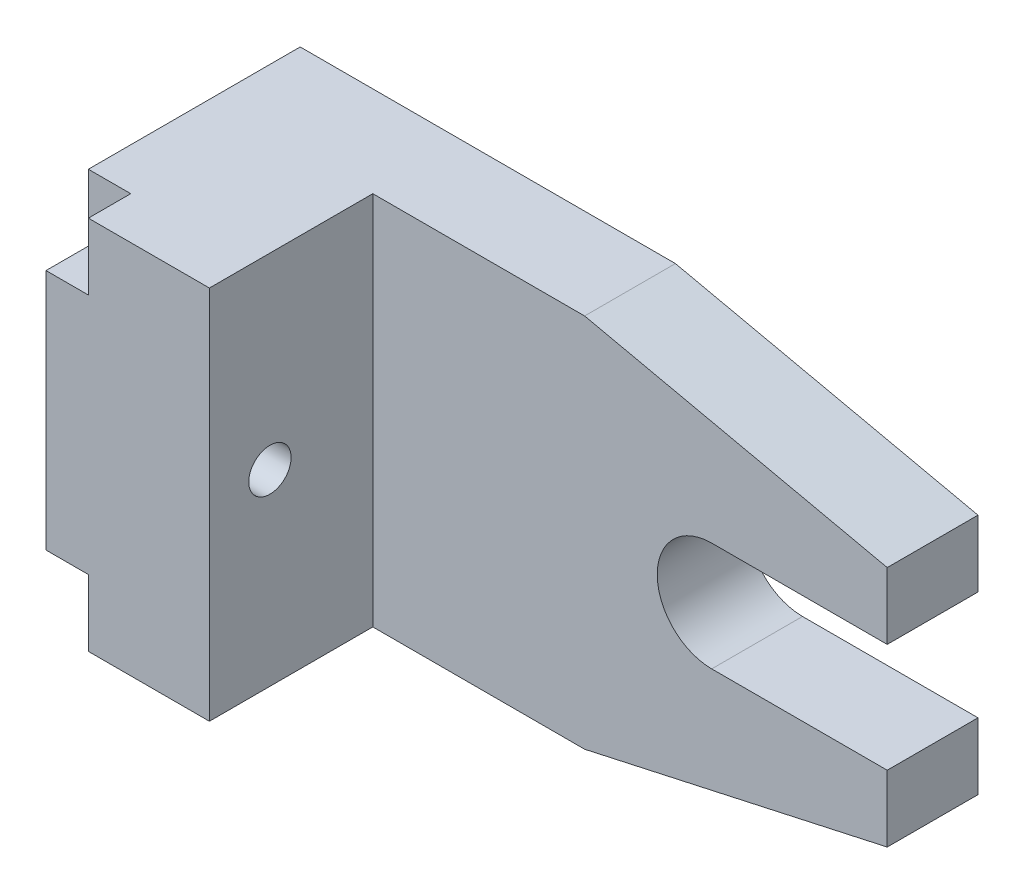
ISO-10303-21;
HEADER;
FILE_DESCRIPTION(('STEP AP214'),'2;1');
FILE_NAME('part.step','',(''),(''),'','','');
FILE_SCHEMA(('AUTOMOTIVE_DESIGN { 1 0 10303 214 1 1 1 1 }'));
ENDSEC;
DATA;
#1=APPLICATION_CONTEXT('core data for automotive mechanical design processes');
#2=APPLICATION_PROTOCOL_DEFINITION('international standard','automotive_design',2000,#1);
#3=PRODUCT_CONTEXT('',#1,'mechanical');
#4=PRODUCT('Part','Part','',(#3));
#5=PRODUCT_RELATED_PRODUCT_CATEGORY('part','',(#4));
#6=PRODUCT_DEFINITION_FORMATION('','',#4);
#7=PRODUCT_DEFINITION_CONTEXT('part definition',#1,'design');
#8=PRODUCT_DEFINITION('design','',#6,#7);
#9=PRODUCT_DEFINITION_SHAPE('','',#8);
#10=(LENGTH_UNIT() NAMED_UNIT(*) SI_UNIT(.MILLI.,.METRE.));
#11=(NAMED_UNIT(*) PLANE_ANGLE_UNIT() SI_UNIT($,.RADIAN.));
#12=(NAMED_UNIT(*) SI_UNIT($,.STERADIAN.) SOLID_ANGLE_UNIT());
#13=UNCERTAINTY_MEASURE_WITH_UNIT(LENGTH_MEASURE(1.E-05),#10,'distance_accuracy_value','');
#14=(GEOMETRIC_REPRESENTATION_CONTEXT(3) GLOBAL_UNCERTAINTY_ASSIGNED_CONTEXT((#13)) GLOBAL_UNIT_ASSIGNED_CONTEXT((#10,
#11,#12)) REPRESENTATION_CONTEXT('',''));
#15=CARTESIAN_POINT('',(0.,0.,0.));
#16=DIRECTION('',(0.,0.,1.));
#17=DIRECTION('',(1.,0.,0.));
#18=AXIS2_PLACEMENT_3D('',#15,#16,#17);
#19=CARTESIAN_POINT('',(0.,62.,15.));
#20=DIRECTION('',(0.,1.,0.));
#21=DIRECTION('',(0.,0.,1.));
#22=AXIS2_PLACEMENT_3D('',#19,#20,#21);
#23=PLANE('',#22);
#24=DIRECTION('',(0.,0.,-1.));
#25=VECTOR('',#24,1.);
#26=CARTESIAN_POINT('',(-27.,62.,42.));
#27=LINE('',#26,#25);
#28=CARTESIAN_POINT('',(-27.,62.,35.));
#29=VERTEX_POINT('',#28);
#30=CARTESIAN_POINT('',(-27.,62.,0.));
#31=VERTEX_POINT('',#30);
#32=EDGE_CURVE('E239',#29,#31,#27,.T.);
#33=ORIENTED_EDGE('',*,*,#32,.F.);
#34=DIRECTION('',(-1.,0.,0.));
#35=VECTOR('',#34,1.);
#36=CARTESIAN_POINT('',(-20.,62.,35.));
#37=LINE('',#36,#35);
#38=CARTESIAN_POINT('',(-20.,62.,35.));
#39=VERTEX_POINT('',#38);
#40=EDGE_CURVE('E196',#39,#29,#37,.T.);
#41=ORIENTED_EDGE('',*,*,#40,.F.);
#42=DIRECTION('',(0.,0.,-1.));
#43=VECTOR('',#42,1.);
#44=CARTESIAN_POINT('',(-20.,62.,0.));
#45=LINE('',#44,#43);
#46=CARTESIAN_POINT('',(-20.,62.,42.));
#47=VERTEX_POINT('',#46);
#48=EDGE_CURVE('E181',#47,#39,#45,.T.);
#49=ORIENTED_EDGE('',*,*,#48,.F.);
#50=DIRECTION('',(-1.,0.,0.));
#51=VECTOR('',#50,1.);
#52=CARTESIAN_POINT('',(0.,62.,42.));
#53=LINE('',#52,#51);
#54=CARTESIAN_POINT('',(0.,62.,42.));
#55=VERTEX_POINT('',#54);
#56=EDGE_CURVE('E221',#55,#47,#53,.T.);
#57=ORIENTED_EDGE('',*,*,#56,.F.);
#58=DIRECTION('',(0.,0.,-1.));
#59=VECTOR('',#58,1.);
#60=CARTESIAN_POINT('',(0.,62.,42.));
#61=LINE('',#60,#59);
#62=CARTESIAN_POINT('',(0.,62.,15.));
#63=VERTEX_POINT('',#62);
#64=EDGE_CURVE('E241',#55,#63,#61,.T.);
#65=ORIENTED_EDGE('',*,*,#64,.T.);
#66=DIRECTION('',(1.,0.,0.));
#67=VECTOR('',#66,1.);
#68=CARTESIAN_POINT('',(0.,62.,15.));
#69=LINE('',#68,#67);
#70=CARTESIAN_POINT('',(35.,62.,15.));
#71=VERTEX_POINT('',#70);
#72=EDGE_CURVE('E258',#63,#71,#69,.T.);
#73=ORIENTED_EDGE('',*,*,#72,.T.);
#74=DIRECTION('',(0.,0.,-1.));
#75=VECTOR('',#74,1.);
#76=CARTESIAN_POINT('',(35.,62.,15.));
#77=LINE('',#76,#75);
#78=CARTESIAN_POINT('',(35.,62.,0.));
#79=VERTEX_POINT('',#78);
#80=EDGE_CURVE('E303',#71,#79,#77,.T.);
#81=ORIENTED_EDGE('',*,*,#80,.T.);
#82=DIRECTION('',(1.,0.,0.));
#83=VECTOR('',#82,1.);
#84=CARTESIAN_POINT('',(0.,62.,0.));
#85=LINE('',#84,#83);
#86=EDGE_CURVE('E282',#31,#79,#85,.T.);
#87=ORIENTED_EDGE('',*,*,#86,.F.);
#88=EDGE_LOOP('',(#33,#41,#49,#57,#65,#73,#81,#87));
#89=FACE_BOUND('',#88,.T.);
#90=ADVANCED_FACE('F45',(#89),#23,.T.);
#91=CARTESIAN_POINT('',(0.,0.,15.));
#92=DIRECTION('',(0.,1.,0.));
#93=DIRECTION('',(0.,0.,1.));
#94=AXIS2_PLACEMENT_3D('',#91,#92,#93);
#95=PLANE('',#94);
#96=DIRECTION('',(-1.,0.,0.));
#97=VECTOR('',#96,1.);
#98=CARTESIAN_POINT('',(-20.,0.,35.));
#99=LINE('',#98,#97);
#100=CARTESIAN_POINT('',(-20.,0.,35.));
#101=VERTEX_POINT('',#100);
#102=CARTESIAN_POINT('',(-27.,0.,35.));
#103=VERTEX_POINT('',#102);
#104=EDGE_CURVE('E220',#101,#103,#99,.T.);
#105=ORIENTED_EDGE('',*,*,#104,.T.);
#106=DIRECTION('',(0.,0.,-1.));
#107=VECTOR('',#106,1.);
#108=CARTESIAN_POINT('',(-27.,0.,42.));
#109=LINE('',#108,#107);
#110=CARTESIAN_POINT('',(-27.,0.,0.));
#111=VERTEX_POINT('',#110);
#112=EDGE_CURVE('E240',#103,#111,#109,.T.);
#113=ORIENTED_EDGE('',*,*,#112,.T.);
#114=DIRECTION('',(1.,0.,0.));
#115=VECTOR('',#114,1.);
#116=CARTESIAN_POINT('',(0.,0.,0.));
#117=LINE('',#116,#115);
#118=CARTESIAN_POINT('',(35.,0.,0.));
#119=VERTEX_POINT('',#118);
#120=EDGE_CURVE('E285',#111,#119,#117,.T.);
#121=ORIENTED_EDGE('',*,*,#120,.T.);
#122=DIRECTION('',(0.,0.,-1.));
#123=VECTOR('',#122,1.);
#124=CARTESIAN_POINT('',(35.,0.,15.));
#125=LINE('',#124,#123);
#126=CARTESIAN_POINT('',(35.,0.,15.));
#127=VERTEX_POINT('',#126);
#128=EDGE_CURVE('E300',#127,#119,#125,.T.);
#129=ORIENTED_EDGE('',*,*,#128,.F.);
#130=DIRECTION('',(1.,0.,0.));
#131=VECTOR('',#130,1.);
#132=CARTESIAN_POINT('',(0.,0.,15.));
#133=LINE('',#132,#131);
#134=CARTESIAN_POINT('',(0.,0.,15.));
#135=VERTEX_POINT('',#134);
#136=EDGE_CURVE('E265',#135,#127,#133,.T.);
#137=ORIENTED_EDGE('',*,*,#136,.F.);
#138=DIRECTION('',(0.,0.,-1.));
#139=VECTOR('',#138,1.);
#140=CARTESIAN_POINT('',(0.,0.,42.));
#141=LINE('',#140,#139);
#142=CARTESIAN_POINT('',(0.,0.,42.));
#143=VERTEX_POINT('',#142);
#144=EDGE_CURVE('E235',#143,#135,#141,.T.);
#145=ORIENTED_EDGE('',*,*,#144,.F.);
#146=DIRECTION('',(1.,0.,0.));
#147=VECTOR('',#146,1.);
#148=CARTESIAN_POINT('',(-27.,0.,42.));
#149=LINE('',#148,#147);
#150=CARTESIAN_POINT('',(-20.,0.,42.));
#151=VERTEX_POINT('',#150);
#152=EDGE_CURVE('E230',#151,#143,#149,.T.);
#153=ORIENTED_EDGE('',*,*,#152,.F.);
#154=DIRECTION('',(0.,0.,1.));
#155=VECTOR('',#154,1.);
#156=CARTESIAN_POINT('',(-20.,0.,0.));
#157=LINE('',#156,#155);
#158=EDGE_CURVE('E67',#101,#151,#157,.T.);
#159=ORIENTED_EDGE('',*,*,#158,.F.);
#160=EDGE_LOOP('',(#105,#113,#121,#129,#137,#145,#153,#159));
#161=FACE_BOUND('',#160,.T.);
#162=ADVANCED_FACE('F342',(#161),#95,.F.);
#163=CARTESIAN_POINT('',(-27.,62.,42.));
#164=DIRECTION('',(1.,0.,0.));
#165=DIRECTION('',(0.,0.,-1.));
#166=AXIS2_PLACEMENT_3D('',#163,#164,#165);
#167=PLANE('',#166);
#168=CARTESIAN_POINT('',(-27.,31.,32.));
#169=DIRECTION('',(-1.,0.,0.));
#170=DIRECTION('',(0.,0.,1.));
#171=AXIS2_PLACEMENT_3D('',#168,#169,#170);
#172=CIRCLE('',#171,3.5);
#173=CARTESIAN_POINT('',(-27.,31.,35.5));
#174=VERTEX_POINT('',#173);
#175=EDGE_CURVE('E195',#174,#174,#172,.T.);
#176=ORIENTED_EDGE('',*,*,#175,.F.);
#177=EDGE_LOOP('',(#176));
#178=FACE_BOUND('',#177,.T.);
#179=DIRECTION('',(0.,1.,0.));
#180=VECTOR('',#179,1.);
#181=CARTESIAN_POINT('',(-27.,0.,35.));
#182=LINE('',#181,#180);
#183=CARTESIAN_POINT('',(-27.,51.,35.));
#184=VERTEX_POINT('',#183);
#185=EDGE_CURVE('E182',#184,#29,#182,.T.);
#186=ORIENTED_EDGE('',*,*,#185,.T.);
#187=ORIENTED_EDGE('',*,*,#32,.T.);
#188=DIRECTION('',(0.,-1.,0.));
#189=VECTOR('',#188,1.);
#190=CARTESIAN_POINT('',(-27.,62.,0.));
#191=LINE('',#190,#189);
#192=EDGE_CURVE('E199',#31,#111,#191,.T.);
#193=ORIENTED_EDGE('',*,*,#192,.T.);
#194=ORIENTED_EDGE('',*,*,#112,.F.);
#195=DIRECTION('',(0.,1.,0.));
#196=VECTOR('',#195,1.);
#197=CARTESIAN_POINT('',(-27.,0.,35.));
#198=LINE('',#197,#196);
#199=CARTESIAN_POINT('',(-27.,11.,35.));
#200=VERTEX_POINT('',#199);
#201=EDGE_CURVE('E202',#103,#200,#198,.T.);
#202=ORIENTED_EDGE('',*,*,#201,.T.);
#203=DIRECTION('',(0.,0.,1.));
#204=VECTOR('',#203,1.);
#205=CARTESIAN_POINT('',(-27.,11.,0.));
#206=LINE('',#205,#204);
#207=CARTESIAN_POINT('',(-27.,11.,42.));
#208=VERTEX_POINT('',#207);
#209=EDGE_CURVE('E211',#200,#208,#206,.T.);
#210=ORIENTED_EDGE('',*,*,#209,.T.);
#211=DIRECTION('',(0.,-1.,0.));
#212=VECTOR('',#211,1.);
#213=CARTESIAN_POINT('',(-27.,62.,42.));
#214=LINE('',#213,#212);
#215=CARTESIAN_POINT('',(-27.,51.,42.));
#216=VERTEX_POINT('',#215);
#217=EDGE_CURVE('E227',#216,#208,#214,.T.);
#218=ORIENTED_EDGE('',*,*,#217,.F.);
#219=DIRECTION('',(0.,0.,-1.));
#220=VECTOR('',#219,1.);
#221=CARTESIAN_POINT('',(-27.,51.,0.));
#222=LINE('',#221,#220);
#223=EDGE_CURVE('E189',#216,#184,#222,.T.);
#224=ORIENTED_EDGE('',*,*,#223,.T.);
#225=EDGE_LOOP('',(#186,#187,#193,#194,#202,#210,#218,#224));
#226=FACE_BOUND('',#225,.T.);
#227=ADVANCED_FACE('F367',(#178,#226),#167,.F.);
#228=CARTESIAN_POINT('',(0.,0.,42.));
#229=DIRECTION('',(0.,0.,1.));
#230=DIRECTION('',(1.,0.,0.));
#231=AXIS2_PLACEMENT_3D('',#228,#229,#230);
#232=PLANE('',#231);
#233=DIRECTION('',(0.,1.,0.));
#234=VECTOR('',#233,1.);
#235=CARTESIAN_POINT('',(-20.,0.,42.));
#236=LINE('',#235,#234);
#237=CARTESIAN_POINT('',(-20.,51.,42.));
#238=VERTEX_POINT('',#237);
#239=EDGE_CURVE('E173',#238,#47,#236,.T.);
#240=ORIENTED_EDGE('',*,*,#239,.F.);
#241=DIRECTION('',(-1.,0.,0.));
#242=VECTOR('',#241,1.);
#243=CARTESIAN_POINT('',(-20.,51.,42.));
#244=LINE('',#243,#242);
#245=EDGE_CURVE('E172',#238,#216,#244,.T.);
#246=ORIENTED_EDGE('',*,*,#245,.T.);
#247=ORIENTED_EDGE('',*,*,#217,.T.);
#248=DIRECTION('',(-1.,0.,0.));
#249=VECTOR('',#248,1.);
#250=CARTESIAN_POINT('',(-20.,11.,42.));
#251=LINE('',#250,#249);
#252=CARTESIAN_POINT('',(-20.,11.,42.));
#253=VERTEX_POINT('',#252);
#254=EDGE_CURVE('E198',#253,#208,#251,.T.);
#255=ORIENTED_EDGE('',*,*,#254,.F.);
#256=DIRECTION('',(0.,1.,0.));
#257=VECTOR('',#256,1.);
#258=CARTESIAN_POINT('',(-20.,0.,42.));
#259=LINE('',#258,#257);
#260=EDGE_CURVE('E208',#151,#253,#259,.T.);
#261=ORIENTED_EDGE('',*,*,#260,.F.);
#262=ORIENTED_EDGE('',*,*,#152,.T.);
#263=DIRECTION('',(0.,1.,0.));
#264=VECTOR('',#263,1.);
#265=CARTESIAN_POINT('',(0.,62.,42.));
#266=LINE('',#265,#264);
#267=EDGE_CURVE('E222',#143,#55,#266,.T.);
#268=ORIENTED_EDGE('',*,*,#267,.T.);
#269=ORIENTED_EDGE('',*,*,#56,.T.);
#270=EDGE_LOOP('',(#240,#246,#247,#255,#261,#262,#268,#269));
#271=FACE_BOUND('',#270,.T.);
#272=ADVANCED_FACE('F361',(#271),#232,.T.);
#273=CARTESIAN_POINT('',(56.,31.,15.));
#274=DIRECTION('',(0.,0.,-1.));
#275=DIRECTION('',(-1.,0.,0.));
#276=AXIS2_PLACEMENT_3D('',#273,#274,#275);
#277=CYLINDRICAL_SURFACE('',#276,8.99999999999999);
#278=CARTESIAN_POINT('',(56.,31.,0.));
#279=DIRECTION('',(0.,0.,1.));
#280=DIRECTION('',(1.,0.,0.));
#281=AXIS2_PLACEMENT_3D('',#278,#279,#280);
#282=CIRCLE('',#281,8.99999999999999);
#283=CARTESIAN_POINT('',(56.,40.,0.));
#284=VERTEX_POINT('',#283);
#285=CARTESIAN_POINT('',(56.,22.,0.));
#286=VERTEX_POINT('',#285);
#287=EDGE_CURVE('E243',#284,#286,#282,.T.);
#288=ORIENTED_EDGE('',*,*,#287,.F.);
#289=DIRECTION('',(0.,0.,-1.));
#290=VECTOR('',#289,1.);
#291=CARTESIAN_POINT('',(56.,40.,15.));
#292=LINE('',#291,#290);
#293=CARTESIAN_POINT('',(56.,40.,15.));
#294=VERTEX_POINT('',#293);
#295=EDGE_CURVE('E12',#294,#284,#292,.T.);
#296=ORIENTED_EDGE('',*,*,#295,.F.);
#297=CARTESIAN_POINT('',(56.,31.,15.));
#298=DIRECTION('',(0.,0.,1.));
#299=DIRECTION('',(1.,0.,0.));
#300=AXIS2_PLACEMENT_3D('',#297,#298,#299);
#301=CIRCLE('',#300,8.99999999999999);
#302=CARTESIAN_POINT('',(56.,22.,15.));
#303=VERTEX_POINT('',#302);
#304=EDGE_CURVE('E245',#294,#303,#301,.T.);
#305=ORIENTED_EDGE('',*,*,#304,.T.);
#306=DIRECTION('',(0.,0.,-1.));
#307=VECTOR('',#306,1.);
#308=CARTESIAN_POINT('',(56.,22.,15.));
#309=LINE('',#308,#307);
#310=EDGE_CURVE('E271',#303,#286,#309,.T.);
#311=ORIENTED_EDGE('',*,*,#310,.T.);
#312=EDGE_LOOP('',(#288,#296,#305,#311));
#313=FACE_BOUND('',#312,.T.);
#314=ADVANCED_FACE('F42',(#313),#277,.F.);
#315=CARTESIAN_POINT('',(0.,40.,15.));
#316=DIRECTION('',(0.,1.,0.));
#317=DIRECTION('',(0.,0.,1.));
#318=AXIS2_PLACEMENT_3D('',#315,#316,#317);
#319=PLANE('',#318);
#320=DIRECTION('',(1.,0.,0.));
#321=VECTOR('',#320,1.);
#322=CARTESIAN_POINT('',(0.,40.,0.));
#323=LINE('',#322,#321);
#324=CARTESIAN_POINT('',(85.,40.,0.));
#325=VERTEX_POINT('',#324);
#326=EDGE_CURVE('E273',#284,#325,#323,.T.);
#327=ORIENTED_EDGE('',*,*,#326,.T.);
#328=DIRECTION('',(0.,0.,-1.));
#329=VECTOR('',#328,1.);
#330=CARTESIAN_POINT('',(85.,40.,15.));
#331=LINE('',#330,#329);
#332=CARTESIAN_POINT('',(85.,40.,15.));
#333=VERTEX_POINT('',#332);
#334=EDGE_CURVE('E51',#333,#325,#331,.T.);
#335=ORIENTED_EDGE('',*,*,#334,.F.);
#336=DIRECTION('',(1.,0.,0.));
#337=VECTOR('',#336,1.);
#338=CARTESIAN_POINT('',(0.,40.,15.));
#339=LINE('',#338,#337);
#340=EDGE_CURVE('E248',#294,#333,#339,.T.);
#341=ORIENTED_EDGE('',*,*,#340,.F.);
#342=ORIENTED_EDGE('',*,*,#295,.T.);
#343=EDGE_LOOP('',(#327,#335,#341,#342));
#344=FACE_BOUND('',#343,.T.);
#345=ADVANCED_FACE('F357',(#344),#319,.F.);
#346=CARTESIAN_POINT('',(85.,0.,15.));
#347=DIRECTION('',(-1.,0.,0.));
#348=DIRECTION('',(0.,0.,1.));
#349=AXIS2_PLACEMENT_3D('',#346,#347,#348);
#350=PLANE('',#349);
#351=DIRECTION('',(0.,1.,0.));
#352=VECTOR('',#351,1.);
#353=CARTESIAN_POINT('',(85.,0.,0.));
#354=LINE('',#353,#352);
#355=CARTESIAN_POINT('',(85.,51.,0.));
#356=VERTEX_POINT('',#355);
#357=EDGE_CURVE('E277',#325,#356,#354,.T.);
#358=ORIENTED_EDGE('',*,*,#357,.T.);
#359=DIRECTION('',(0.,0.,-1.));
#360=VECTOR('',#359,1.);
#361=CARTESIAN_POINT('',(85.,51.,15.));
#362=LINE('',#361,#360);
#363=CARTESIAN_POINT('',(85.,51.,15.));
#364=VERTEX_POINT('',#363);
#365=EDGE_CURVE('E301',#364,#356,#362,.T.);
#366=ORIENTED_EDGE('',*,*,#365,.F.);
#367=DIRECTION('',(0.,1.,0.));
#368=VECTOR('',#367,1.);
#369=CARTESIAN_POINT('',(85.,0.,15.));
#370=LINE('',#369,#368);
#371=EDGE_CURVE('E253',#333,#364,#370,.T.);
#372=ORIENTED_EDGE('',*,*,#371,.F.);
#373=ORIENTED_EDGE('',*,*,#334,.T.);
#374=EDGE_LOOP('',(#358,#366,#372,#373));
#375=FACE_BOUND('',#374,.T.);
#376=ADVANCED_FACE('F315',(#375),#350,.F.);
#377=CARTESIAN_POINT('',(14.6260969095765,66.4822586798932,15.));
#378=DIRECTION('',(0.21486178267512,0.97664446670509,0.));
#379=DIRECTION('',(-0.97664446670509,0.21486178267512,0.));
#380=AXIS2_PLACEMENT_3D('',#377,#378,#379);
#381=PLANE('',#380);
#382=DIRECTION('',(0.97664446670509,-0.21486178267512,0.));
#383=VECTOR('',#382,1.);
#384=CARTESIAN_POINT('',(14.6260969095765,66.4822586798932,0.));
#385=LINE('',#384,#383);
#386=EDGE_CURVE('E276',#79,#356,#385,.T.);
#387=ORIENTED_EDGE('',*,*,#386,.F.);
#388=ORIENTED_EDGE('',*,*,#80,.F.);
#389=DIRECTION('',(0.97664446670509,-0.21486178267512,0.));
#390=VECTOR('',#389,1.);
#391=CARTESIAN_POINT('',(14.6260969095765,66.4822586798932,15.));
#392=LINE('',#391,#390);
#393=EDGE_CURVE('E251',#71,#364,#392,.T.);
#394=ORIENTED_EDGE('',*,*,#393,.T.);
#395=ORIENTED_EDGE('',*,*,#365,.T.);
#396=EDGE_LOOP('',(#387,#388,#394,#395));
#397=FACE_BOUND('',#396,.T.);
#398=ADVANCED_FACE('F322',(#397),#381,.T.);
#399=CARTESIAN_POINT('',(1.61579549790156,-7.34452499046166,15.));
#400=DIRECTION('',(-0.21486178267512,0.97664446670509,0.));
#401=DIRECTION('',(-0.97664446670509,-0.21486178267512,0.));
#402=AXIS2_PLACEMENT_3D('',#399,#400,#401);
#403=PLANE('',#402);
#404=DIRECTION('',(0.97664446670509,0.21486178267512,0.));
#405=VECTOR('',#404,1.);
#406=CARTESIAN_POINT('',(1.61579549790156,-7.34452499046166,0.));
#407=LINE('',#406,#405);
#408=CARTESIAN_POINT('',(85.,11.,0.));
#409=VERTEX_POINT('',#408);
#410=EDGE_CURVE('E290',#119,#409,#407,.T.);
#411=ORIENTED_EDGE('',*,*,#410,.T.);
#412=DIRECTION('',(0.,0.,-1.));
#413=VECTOR('',#412,1.);
#414=CARTESIAN_POINT('',(85.,11.,15.));
#415=LINE('',#414,#413);
#416=CARTESIAN_POINT('',(85.,11.,15.));
#417=VERTEX_POINT('',#416);
#418=EDGE_CURVE('E297',#417,#409,#415,.T.);
#419=ORIENTED_EDGE('',*,*,#418,.F.);
#420=DIRECTION('',(0.97664446670509,0.21486178267512,0.));
#421=VECTOR('',#420,1.);
#422=CARTESIAN_POINT('',(1.61579549790156,-7.34452499046166,15.));
#423=LINE('',#422,#421);
#424=EDGE_CURVE('E262',#127,#417,#423,.T.);
#425=ORIENTED_EDGE('',*,*,#424,.F.);
#426=ORIENTED_EDGE('',*,*,#128,.T.);
#427=EDGE_LOOP('',(#411,#419,#425,#426));
#428=FACE_BOUND('',#427,.T.);
#429=ADVANCED_FACE('F341',(#428),#403,.F.);
#430=CARTESIAN_POINT('',(85.,1.07237451242203E-13,15.));
#431=DIRECTION('',(-1.,0.,0.));
#432=DIRECTION('',(0.,-1.,0.));
#433=AXIS2_PLACEMENT_3D('',#430,#431,#432);
#434=PLANE('',#433);
#435=DIRECTION('',(0.,1.,0.));
#436=VECTOR('',#435,1.);
#437=CARTESIAN_POINT('',(85.,1.07237451242203E-13,0.));
#438=LINE('',#437,#436);
#439=CARTESIAN_POINT('',(85.,22.,0.));
#440=VERTEX_POINT('',#439);
#441=EDGE_CURVE('E289',#409,#440,#438,.T.);
#442=ORIENTED_EDGE('',*,*,#441,.T.);
#443=DIRECTION('',(0.,0.,-1.));
#444=VECTOR('',#443,1.);
#445=CARTESIAN_POINT('',(85.,22.,15.));
#446=LINE('',#445,#444);
#447=CARTESIAN_POINT('',(85.,22.,15.));
#448=VERTEX_POINT('',#447);
#449=EDGE_CURVE('E293',#448,#440,#446,.T.);
#450=ORIENTED_EDGE('',*,*,#449,.F.);
#451=DIRECTION('',(0.,1.,0.));
#452=VECTOR('',#451,1.);
#453=CARTESIAN_POINT('',(85.,1.07237451242203E-13,15.));
#454=LINE('',#453,#452);
#455=EDGE_CURVE('E266',#417,#448,#454,.T.);
#456=ORIENTED_EDGE('',*,*,#455,.F.);
#457=ORIENTED_EDGE('',*,*,#418,.T.);
#458=EDGE_LOOP('',(#442,#450,#456,#457));
#459=FACE_BOUND('',#458,.T.);
#460=ADVANCED_FACE('F348',(#459),#434,.F.);
#461=CARTESIAN_POINT('',(0.,22.,15.));
#462=DIRECTION('',(0.,1.,0.));
#463=DIRECTION('',(0.,0.,1.));
#464=AXIS2_PLACEMENT_3D('',#461,#462,#463);
#465=PLANE('',#464);
#466=DIRECTION('',(1.,0.,0.));
#467=VECTOR('',#466,1.);
#468=CARTESIAN_POINT('',(0.,22.,0.));
#469=LINE('',#468,#467);
#470=EDGE_CURVE('E249',#286,#440,#469,.T.);
#471=ORIENTED_EDGE('',*,*,#470,.F.);
#472=ORIENTED_EDGE('',*,*,#310,.F.);
#473=DIRECTION('',(1.,0.,0.));
#474=VECTOR('',#473,1.);
#475=CARTESIAN_POINT('',(0.,22.,15.));
#476=LINE('',#475,#474);
#477=EDGE_CURVE('E268',#303,#448,#476,.T.);
#478=ORIENTED_EDGE('',*,*,#477,.T.);
#479=ORIENTED_EDGE('',*,*,#449,.T.);
#480=EDGE_LOOP('',(#471,#472,#478,#479));
#481=FACE_BOUND('',#480,.T.);
#482=ADVANCED_FACE('F353',(#481),#465,.T.);
#483=CARTESIAN_POINT('',(0.,0.,15.));
#484=DIRECTION('',(0.,0.,1.));
#485=DIRECTION('',(1.,0.,0.));
#486=AXIS2_PLACEMENT_3D('',#483,#484,#485);
#487=PLANE('',#486);
#488=ORIENTED_EDGE('',*,*,#304,.F.);
#489=ORIENTED_EDGE('',*,*,#340,.T.);
#490=ORIENTED_EDGE('',*,*,#371,.T.);
#491=ORIENTED_EDGE('',*,*,#393,.F.);
#492=ORIENTED_EDGE('',*,*,#72,.F.);
#493=DIRECTION('',(0.,1.,0.));
#494=VECTOR('',#493,1.);
#495=CARTESIAN_POINT('',(0.,0.,15.));
#496=LINE('',#495,#494);
#497=EDGE_CURVE('E259',#135,#63,#496,.T.);
#498=ORIENTED_EDGE('',*,*,#497,.F.);
#499=ORIENTED_EDGE('',*,*,#136,.T.);
#500=ORIENTED_EDGE('',*,*,#424,.T.);
#501=ORIENTED_EDGE('',*,*,#455,.T.);
#502=ORIENTED_EDGE('',*,*,#477,.F.);
#503=EDGE_LOOP('',(#488,#489,#490,#491,#492,#498,#499,#500,#501,#502));
#504=FACE_BOUND('',#503,.T.);
#505=ADVANCED_FACE('F327',(#504),#487,.T.);
#506=CARTESIAN_POINT('',(0.,0.,0.));
#507=DIRECTION('',(0.,0.,1.));
#508=DIRECTION('',(1.,0.,0.));
#509=AXIS2_PLACEMENT_3D('',#506,#507,#508);
#510=PLANE('',#509);
#511=ORIENTED_EDGE('',*,*,#287,.T.);
#512=ORIENTED_EDGE('',*,*,#470,.T.);
#513=ORIENTED_EDGE('',*,*,#441,.F.);
#514=ORIENTED_EDGE('',*,*,#410,.F.);
#515=ORIENTED_EDGE('',*,*,#120,.F.);
#516=ORIENTED_EDGE('',*,*,#192,.F.);
#517=ORIENTED_EDGE('',*,*,#86,.T.);
#518=ORIENTED_EDGE('',*,*,#386,.T.);
#519=ORIENTED_EDGE('',*,*,#357,.F.);
#520=ORIENTED_EDGE('',*,*,#326,.F.);
#521=EDGE_LOOP('',(#511,#512,#513,#514,#515,#516,#517,#518,#519,#520));
#522=FACE_BOUND('',#521,.T.);
#523=ADVANCED_FACE('F318',(#522),#510,.F.);
#524=CARTESIAN_POINT('',(0.,62.,42.));
#525=DIRECTION('',(-1.,0.,0.));
#526=DIRECTION('',(0.,0.,1.));
#527=AXIS2_PLACEMENT_3D('',#524,#525,#526);
#528=PLANE('',#527);
#529=CARTESIAN_POINT('',(0.,31.,32.));
#530=DIRECTION('',(-1.,0.,0.));
#531=DIRECTION('',(0.,0.,1.));
#532=AXIS2_PLACEMENT_3D('',#529,#530,#531);
#533=CIRCLE('',#532,3.5);
#534=CARTESIAN_POINT('',(0.,31.,35.5));
#535=VERTEX_POINT('',#534);
#536=EDGE_CURVE('E46',#535,#535,#533,.T.);
#537=ORIENTED_EDGE('',*,*,#536,.T.);
#538=EDGE_LOOP('',(#537));
#539=FACE_BOUND('',#538,.T.);
#540=ORIENTED_EDGE('',*,*,#144,.T.);
#541=ORIENTED_EDGE('',*,*,#497,.T.);
#542=ORIENTED_EDGE('',*,*,#64,.F.);
#543=ORIENTED_EDGE('',*,*,#267,.F.);
#544=EDGE_LOOP('',(#540,#541,#542,#543));
#545=FACE_BOUND('',#544,.T.);
#546=ADVANCED_FACE('F333',(#539,#545),#528,.F.);
#547=CARTESIAN_POINT('',(-20.,11.,0.));
#548=DIRECTION('',(0.,-1.,0.));
#549=DIRECTION('',(0.,0.,-1.));
#550=AXIS2_PLACEMENT_3D('',#547,#548,#549);
#551=PLANE('',#550);
#552=ORIENTED_EDGE('',*,*,#209,.F.);
#553=DIRECTION('',(-1.,0.,0.));
#554=VECTOR('',#553,1.);
#555=CARTESIAN_POINT('',(-20.,11.,35.));
#556=LINE('',#555,#554);
#557=CARTESIAN_POINT('',(-20.,11.,35.));
#558=VERTEX_POINT('',#557);
#559=EDGE_CURVE('E209',#558,#200,#556,.T.);
#560=ORIENTED_EDGE('',*,*,#559,.F.);
#561=DIRECTION('',(0.,0.,1.));
#562=VECTOR('',#561,1.);
#563=CARTESIAN_POINT('',(-20.,11.,0.));
#564=LINE('',#563,#562);
#565=EDGE_CURVE('E205',#558,#253,#564,.T.);
#566=ORIENTED_EDGE('',*,*,#565,.T.);
#567=ORIENTED_EDGE('',*,*,#254,.T.);
#568=EDGE_LOOP('',(#552,#560,#566,#567));
#569=FACE_BOUND('',#568,.T.);
#570=ADVANCED_FACE('F388',(#569),#551,.T.);
#571=CARTESIAN_POINT('',(-20.,0.,35.));
#572=DIRECTION('',(0.,0.,1.));
#573=DIRECTION('',(1.,0.,0.));
#574=AXIS2_PLACEMENT_3D('',#571,#572,#573);
#575=PLANE('',#574);
#576=ORIENTED_EDGE('',*,*,#201,.F.);
#577=ORIENTED_EDGE('',*,*,#104,.F.);
#578=DIRECTION('',(0.,1.,0.));
#579=VECTOR('',#578,1.);
#580=CARTESIAN_POINT('',(-20.,0.,35.));
#581=LINE('',#580,#579);
#582=EDGE_CURVE('E204',#101,#558,#581,.T.);
#583=ORIENTED_EDGE('',*,*,#582,.T.);
#584=ORIENTED_EDGE('',*,*,#559,.T.);
#585=EDGE_LOOP('',(#576,#577,#583,#584));
#586=FACE_BOUND('',#585,.T.);
#587=ADVANCED_FACE('F396',(#586),#575,.T.);
#588=CARTESIAN_POINT('',(-20.,0.,0.));
#589=DIRECTION('',(-1.,0.,0.));
#590=DIRECTION('',(0.,0.,1.));
#591=AXIS2_PLACEMENT_3D('',#588,#589,#590);
#592=PLANE('',#591);
#593=ORIENTED_EDGE('',*,*,#565,.F.);
#594=ORIENTED_EDGE('',*,*,#582,.F.);
#595=ORIENTED_EDGE('',*,*,#158,.T.);
#596=ORIENTED_EDGE('',*,*,#260,.T.);
#597=EDGE_LOOP('',(#593,#594,#595,#596));
#598=FACE_BOUND('',#597,.T.);
#599=ADVANCED_FACE('F404',(#598),#592,.T.);
#600=CARTESIAN_POINT('',(-20.,0.,35.));
#601=DIRECTION('',(0.,0.,1.));
#602=DIRECTION('',(1.,0.,0.));
#603=AXIS2_PLACEMENT_3D('',#600,#601,#602);
#604=PLANE('',#603);
#605=ORIENTED_EDGE('',*,*,#185,.F.);
#606=DIRECTION('',(-1.,0.,0.));
#607=VECTOR('',#606,1.);
#608=CARTESIAN_POINT('',(-20.,51.,35.));
#609=LINE('',#608,#607);
#610=CARTESIAN_POINT('',(-20.,51.,35.));
#611=VERTEX_POINT('',#610);
#612=EDGE_CURVE('E166',#611,#184,#609,.T.);
#613=ORIENTED_EDGE('',*,*,#612,.F.);
#614=DIRECTION('',(0.,1.,0.));
#615=VECTOR('',#614,1.);
#616=CARTESIAN_POINT('',(-20.,0.,35.));
#617=LINE('',#616,#615);
#618=EDGE_CURVE('E175',#611,#39,#617,.T.);
#619=ORIENTED_EDGE('',*,*,#618,.T.);
#620=ORIENTED_EDGE('',*,*,#40,.T.);
#621=EDGE_LOOP('',(#605,#613,#619,#620));
#622=FACE_BOUND('',#621,.T.);
#623=ADVANCED_FACE('F178',(#622),#604,.T.);
#624=CARTESIAN_POINT('',(-20.,51.,0.));
#625=DIRECTION('',(0.,1.,0.));
#626=DIRECTION('',(0.,0.,1.));
#627=AXIS2_PLACEMENT_3D('',#624,#625,#626);
#628=PLANE('',#627);
#629=ORIENTED_EDGE('',*,*,#223,.F.);
#630=ORIENTED_EDGE('',*,*,#245,.F.);
#631=DIRECTION('',(0.,0.,-1.));
#632=VECTOR('',#631,1.);
#633=CARTESIAN_POINT('',(-20.,51.,0.));
#634=LINE('',#633,#632);
#635=EDGE_CURVE('E59',#238,#611,#634,.T.);
#636=ORIENTED_EDGE('',*,*,#635,.T.);
#637=ORIENTED_EDGE('',*,*,#612,.T.);
#638=EDGE_LOOP('',(#629,#630,#636,#637));
#639=FACE_BOUND('',#638,.T.);
#640=ADVANCED_FACE('F169',(#639),#628,.T.);
#641=CARTESIAN_POINT('',(-20.,0.,0.));
#642=DIRECTION('',(-1.,0.,0.));
#643=DIRECTION('',(0.,0.,1.));
#644=AXIS2_PLACEMENT_3D('',#641,#642,#643);
#645=PLANE('',#644);
#646=ORIENTED_EDGE('',*,*,#618,.F.);
#647=ORIENTED_EDGE('',*,*,#635,.F.);
#648=ORIENTED_EDGE('',*,*,#239,.T.);
#649=ORIENTED_EDGE('',*,*,#48,.T.);
#650=EDGE_LOOP('',(#646,#647,#648,#649));
#651=FACE_BOUND('',#650,.T.);
#652=ADVANCED_FACE('F183',(#651),#645,.T.);
#653=CARTESIAN_POINT('',(85.,31.,32.));
#654=DIRECTION('',(-1.,0.,0.));
#655=DIRECTION('',(0.,0.,1.));
#656=AXIS2_PLACEMENT_3D('',#653,#654,#655);
#657=CYLINDRICAL_SURFACE('',#656,3.5);
#658=ORIENTED_EDGE('',*,*,#175,.T.);
#659=EDGE_LOOP('',(#658));
#660=FACE_BOUND('',#659,.T.);
#661=ORIENTED_EDGE('',*,*,#536,.F.);
#662=EDGE_LOOP('',(#661));
#663=FACE_BOUND('',#662,.T.);
#664=ADVANCED_FACE('F414',(#660,#663),#657,.F.);
#665=CLOSED_SHELL('',(#90,#162,#227,#272,#314,#345,#376,#398,#429,#460,#482,#505,#523,#546,#570,
#587,#599,#623,#640,#652,#664));
#666=MANIFOLD_SOLID_BREP('B2',#665);
#667=ADVANCED_BREP_SHAPE_REPRESENTATION('',(#18,#666),#14);
#668=SHAPE_DEFINITION_REPRESENTATION(#9,#667);
ENDSEC;
END-ISO-10303-21;
